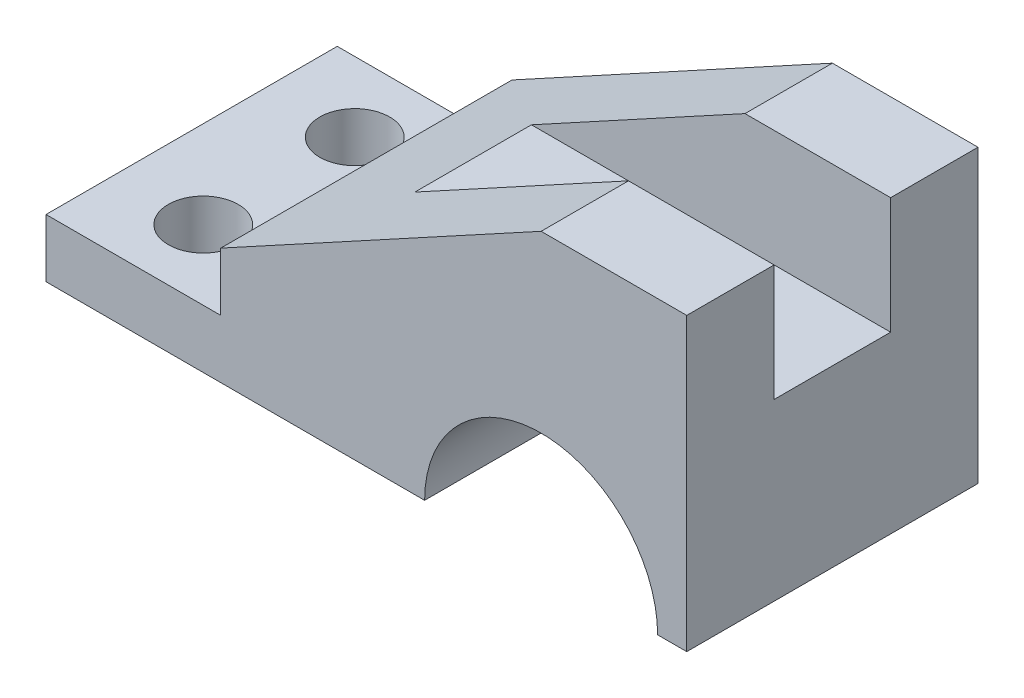
ISO-10303-21;
HEADER;
FILE_DESCRIPTION(('STEP AP214'),'2;1');
FILE_NAME('part.step','',(''),(''),'','','');
FILE_SCHEMA(('AUTOMOTIVE_DESIGN { 1 0 10303 214 1 1 1 1 }'));
ENDSEC;
DATA;
#1=APPLICATION_CONTEXT('core data for automotive mechanical design processes');
#2=APPLICATION_PROTOCOL_DEFINITION('international standard','automotive_design',2000,#1);
#3=PRODUCT_CONTEXT('',#1,'mechanical');
#4=PRODUCT('Part','Part','',(#3));
#5=PRODUCT_RELATED_PRODUCT_CATEGORY('part','',(#4));
#6=PRODUCT_DEFINITION_FORMATION('','',#4);
#7=PRODUCT_DEFINITION_CONTEXT('part definition',#1,'design');
#8=PRODUCT_DEFINITION('design','',#6,#7);
#9=PRODUCT_DEFINITION_SHAPE('','',#8);
#10=(LENGTH_UNIT() NAMED_UNIT(*) SI_UNIT(.MILLI.,.METRE.));
#11=(NAMED_UNIT(*) PLANE_ANGLE_UNIT() SI_UNIT($,.RADIAN.));
#12=(NAMED_UNIT(*) SI_UNIT($,.STERADIAN.) SOLID_ANGLE_UNIT());
#13=UNCERTAINTY_MEASURE_WITH_UNIT(LENGTH_MEASURE(1.E-05),#10,'distance_accuracy_value','');
#14=(GEOMETRIC_REPRESENTATION_CONTEXT(3) GLOBAL_UNCERTAINTY_ASSIGNED_CONTEXT((#13)) GLOBAL_UNIT_ASSIGNED_CONTEXT((#10,
#11,#12)) REPRESENTATION_CONTEXT('',''));
#15=CARTESIAN_POINT('',(0.,0.,0.));
#16=DIRECTION('',(0.,0.,1.));
#17=DIRECTION('',(1.,0.,0.));
#18=AXIS2_PLACEMENT_3D('',#15,#16,#17);
#19=CARTESIAN_POINT('',(110.,50.,50.));
#20=DIRECTION('',(0.,-1.,0.));
#21=DIRECTION('',(0.,0.,-1.));
#22=AXIS2_PLACEMENT_3D('',#19,#20,#21);
#23=PLANE('',#22);
#24=DIRECTION('',(0.,0.,-1.));
#25=VECTOR('',#24,1.);
#26=CARTESIAN_POINT('',(110.,50.,50.));
#27=LINE('',#26,#25);
#28=CARTESIAN_POINT('',(110.,50.,50.));
#29=VERTEX_POINT('',#28);
#30=CARTESIAN_POINT('',(110.,50.,35.));
#31=VERTEX_POINT('',#30);
#32=EDGE_CURVE('E174',#29,#31,#27,.T.);
#33=ORIENTED_EDGE('',*,*,#32,.T.);
#34=DIRECTION('',(1.,0.,0.));
#35=VECTOR('',#34,1.);
#36=CARTESIAN_POINT('',(85.,50.,35.));
#37=LINE('',#36,#35);
#38=CARTESIAN_POINT('',(85.,50.,35.));
#39=VERTEX_POINT('',#38);
#40=EDGE_CURVE('E220',#39,#31,#37,.T.);
#41=ORIENTED_EDGE('',*,*,#40,.F.);
#42=DIRECTION('',(0.,0.,-1.));
#43=VECTOR('',#42,1.);
#44=CARTESIAN_POINT('',(85.,50.,50.));
#45=LINE('',#44,#43);
#46=CARTESIAN_POINT('',(85.,50.,50.));
#47=VERTEX_POINT('',#46);
#48=EDGE_CURVE('E166',#47,#39,#45,.T.);
#49=ORIENTED_EDGE('',*,*,#48,.F.);
#50=DIRECTION('',(-1.,0.,0.));
#51=VECTOR('',#50,1.);
#52=CARTESIAN_POINT('',(110.,50.,50.));
#53=LINE('',#52,#51);
#54=EDGE_CURVE('E126',#29,#47,#53,.T.);
#55=ORIENTED_EDGE('',*,*,#54,.F.);
#56=EDGE_LOOP('',(#33,#41,#49,#55));
#57=FACE_BOUND('',#56,.T.);
#58=ADVANCED_FACE('F39',(#57),#23,.F.);
#59=CARTESIAN_POINT('',(0.,0.,50.));
#60=DIRECTION('',(1.,0.,0.));
#61=DIRECTION('',(0.,0.,-1.));
#62=AXIS2_PLACEMENT_3D('',#59,#60,#61);
#63=PLANE('',#62);
#64=DIRECTION('',(0.,-1.,0.));
#65=VECTOR('',#64,1.);
#66=CARTESIAN_POINT('',(0.,0.,0.));
#67=LINE('',#66,#65);
#68=CARTESIAN_POINT('',(0.,10.,0.));
#69=VERTEX_POINT('',#68);
#70=CARTESIAN_POINT('',(0.,0.,0.));
#71=VERTEX_POINT('',#70);
#72=EDGE_CURVE('E150',#69,#71,#67,.T.);
#73=ORIENTED_EDGE('',*,*,#72,.T.);
#74=DIRECTION('',(0.,0.,-1.));
#75=VECTOR('',#74,1.);
#76=CARTESIAN_POINT('',(0.,0.,50.));
#77=LINE('',#76,#75);
#78=CARTESIAN_POINT('',(0.,0.,50.));
#79=VERTEX_POINT('',#78);
#80=EDGE_CURVE('E11',#79,#71,#77,.T.);
#81=ORIENTED_EDGE('',*,*,#80,.F.);
#82=DIRECTION('',(0.,-1.,0.));
#83=VECTOR('',#82,1.);
#84=CARTESIAN_POINT('',(0.,0.,50.));
#85=LINE('',#84,#83);
#86=CARTESIAN_POINT('',(0.,10.,50.));
#87=VERTEX_POINT('',#86);
#88=EDGE_CURVE('E167',#87,#79,#85,.T.);
#89=ORIENTED_EDGE('',*,*,#88,.F.);
#90=DIRECTION('',(0.,0.,-1.));
#91=VECTOR('',#90,1.);
#92=CARTESIAN_POINT('',(0.,10.,50.));
#93=LINE('',#92,#91);
#94=EDGE_CURVE('E141',#87,#69,#93,.T.);
#95=ORIENTED_EDGE('',*,*,#94,.T.);
#96=EDGE_LOOP('',(#73,#81,#89,#95));
#97=FACE_BOUND('',#96,.T.);
#98=ADVANCED_FACE('F41',(#97),#63,.F.);
#99=CARTESIAN_POINT('',(0.,0.,50.));
#100=DIRECTION('',(0.,1.,0.));
#101=DIRECTION('',(0.,0.,1.));
#102=AXIS2_PLACEMENT_3D('',#99,#100,#101);
#103=PLANE('',#102);
#104=CARTESIAN_POINT('',(15.,0.,12.));
#105=DIRECTION('',(0.,1.,0.));
#106=DIRECTION('',(0.,0.,1.));
#107=AXIS2_PLACEMENT_3D('',#104,#105,#106);
#108=CIRCLE('',#107,6.);
#109=CARTESIAN_POINT('',(15.,0.,18.));
#110=VERTEX_POINT('',#109);
#111=EDGE_CURVE('E239',#110,#110,#108,.T.);
#112=ORIENTED_EDGE('',*,*,#111,.T.);
#113=EDGE_LOOP('',(#112));
#114=FACE_BOUND('',#113,.T.);
#115=CARTESIAN_POINT('',(15.,0.,38.));
#116=DIRECTION('',(0.,1.,0.));
#117=DIRECTION('',(0.,0.,1.));
#118=AXIS2_PLACEMENT_3D('',#115,#116,#117);
#119=CIRCLE('',#118,6.);
#120=CARTESIAN_POINT('',(15.,0.,44.));
#121=VERTEX_POINT('',#120);
#122=EDGE_CURVE('E242',#121,#121,#119,.T.);
#123=ORIENTED_EDGE('',*,*,#122,.T.);
#124=EDGE_LOOP('',(#123));
#125=FACE_BOUND('',#124,.T.);
#126=DIRECTION('',(1.,0.,0.));
#127=VECTOR('',#126,1.);
#128=CARTESIAN_POINT('',(0.,0.,0.));
#129=LINE('',#128,#127);
#130=CARTESIAN_POINT('',(65.,0.,0.));
#131=VERTEX_POINT('',#130);
#132=EDGE_CURVE('E147',#71,#131,#129,.T.);
#133=ORIENTED_EDGE('',*,*,#132,.T.);
#134=DIRECTION('',(0.,0.,-1.));
#135=VECTOR('',#134,1.);
#136=CARTESIAN_POINT('',(65.,0.,50.));
#137=LINE('',#136,#135);
#138=CARTESIAN_POINT('',(65.,0.,50.));
#139=VERTEX_POINT('',#138);
#140=EDGE_CURVE('E48',#139,#131,#137,.T.);
#141=ORIENTED_EDGE('',*,*,#140,.F.);
#142=DIRECTION('',(1.,0.,0.));
#143=VECTOR('',#142,1.);
#144=CARTESIAN_POINT('',(0.,0.,50.));
#145=LINE('',#144,#143);
#146=EDGE_CURVE('E103',#79,#139,#145,.T.);
#147=ORIENTED_EDGE('',*,*,#146,.F.);
#148=ORIENTED_EDGE('',*,*,#80,.T.);
#149=EDGE_LOOP('',(#133,#141,#147,#148));
#150=FACE_BOUND('',#149,.T.);
#151=ADVANCED_FACE('F252',(#114,#125,#150),#103,.F.);
#152=CARTESIAN_POINT('',(85.,0.,50.));
#153=DIRECTION('',(0.,0.,-1.));
#154=DIRECTION('',(-1.,0.,0.));
#155=AXIS2_PLACEMENT_3D('',#152,#153,#154);
#156=CYLINDRICAL_SURFACE('',#155,20.);
#157=CARTESIAN_POINT('',(85.,0.,0.));
#158=DIRECTION('',(0.,0.,-1.));
#159=DIRECTION('',(1.,0.,0.));
#160=AXIS2_PLACEMENT_3D('',#157,#158,#159);
#161=CIRCLE('',#160,20.);
#162=CARTESIAN_POINT('',(105.,0.,0.));
#163=VERTEX_POINT('',#162);
#164=EDGE_CURVE('E153',#131,#163,#161,.T.);
#165=ORIENTED_EDGE('',*,*,#164,.T.);
#166=DIRECTION('',(0.,0.,-1.));
#167=VECTOR('',#166,1.);
#168=CARTESIAN_POINT('',(105.,0.,50.));
#169=LINE('',#168,#167);
#170=CARTESIAN_POINT('',(105.,0.,50.));
#171=VERTEX_POINT('',#170);
#172=EDGE_CURVE('E177',#171,#163,#169,.T.);
#173=ORIENTED_EDGE('',*,*,#172,.F.);
#174=CARTESIAN_POINT('',(85.,0.,50.));
#175=DIRECTION('',(0.,0.,-1.));
#176=DIRECTION('',(1.,0.,0.));
#177=AXIS2_PLACEMENT_3D('',#174,#175,#176);
#178=CIRCLE('',#177,20.);
#179=EDGE_CURVE('E188',#139,#171,#178,.T.);
#180=ORIENTED_EDGE('',*,*,#179,.F.);
#181=ORIENTED_EDGE('',*,*,#140,.T.);
#182=EDGE_LOOP('',(#165,#173,#180,#181));
#183=FACE_BOUND('',#182,.T.);
#184=ADVANCED_FACE('F184',(#183),#156,.F.);
#185=CARTESIAN_POINT('',(105.,0.,50.));
#186=DIRECTION('',(0.,1.,0.));
#187=DIRECTION('',(0.,0.,1.));
#188=AXIS2_PLACEMENT_3D('',#185,#186,#187);
#189=PLANE('',#188);
#190=DIRECTION('',(1.,0.,0.));
#191=VECTOR('',#190,1.);
#192=CARTESIAN_POINT('',(105.,0.,0.));
#193=LINE('',#192,#191);
#194=CARTESIAN_POINT('',(110.,0.,0.));
#195=VERTEX_POINT('',#194);
#196=EDGE_CURVE('E154',#163,#195,#193,.T.);
#197=ORIENTED_EDGE('',*,*,#196,.T.);
#198=DIRECTION('',(0.,0.,-1.));
#199=VECTOR('',#198,1.);
#200=CARTESIAN_POINT('',(110.,0.,50.));
#201=LINE('',#200,#199);
#202=CARTESIAN_POINT('',(110.,0.,50.));
#203=VERTEX_POINT('',#202);
#204=EDGE_CURVE('E171',#203,#195,#201,.T.);
#205=ORIENTED_EDGE('',*,*,#204,.F.);
#206=DIRECTION('',(1.,0.,0.));
#207=VECTOR('',#206,1.);
#208=CARTESIAN_POINT('',(105.,0.,50.));
#209=LINE('',#208,#207);
#210=EDGE_CURVE('E202',#171,#203,#209,.T.);
#211=ORIENTED_EDGE('',*,*,#210,.F.);
#212=ORIENTED_EDGE('',*,*,#172,.T.);
#213=EDGE_LOOP('',(#197,#205,#211,#212));
#214=FACE_BOUND('',#213,.T.);
#215=ADVANCED_FACE('F191',(#214),#189,.F.);
#216=CARTESIAN_POINT('',(110.,0.,50.));
#217=DIRECTION('',(-1.,0.,0.));
#218=DIRECTION('',(0.,0.,1.));
#219=AXIS2_PLACEMENT_3D('',#216,#217,#218);
#220=PLANE('',#219);
#221=DIRECTION('',(0.,0.,-1.));
#222=VECTOR('',#221,1.);
#223=CARTESIAN_POINT('',(110.,30.,15.));
#224=LINE('',#223,#222);
#225=CARTESIAN_POINT('',(110.,30.,35.));
#226=VERTEX_POINT('',#225);
#227=CARTESIAN_POINT('',(110.,30.,15.));
#228=VERTEX_POINT('',#227);
#229=EDGE_CURVE('E219',#226,#228,#224,.T.);
#230=ORIENTED_EDGE('',*,*,#229,.F.);
#231=DIRECTION('',(0.,1.,0.));
#232=VECTOR('',#231,1.);
#233=CARTESIAN_POINT('',(110.,30.,35.));
#234=LINE('',#233,#232);
#235=EDGE_CURVE('E151',#226,#31,#234,.T.);
#236=ORIENTED_EDGE('',*,*,#235,.T.);
#237=ORIENTED_EDGE('',*,*,#32,.F.);
#238=DIRECTION('',(0.,1.,0.));
#239=VECTOR('',#238,1.);
#240=CARTESIAN_POINT('',(110.,0.,50.));
#241=LINE('',#240,#239);
#242=EDGE_CURVE('E201',#203,#29,#241,.T.);
#243=ORIENTED_EDGE('',*,*,#242,.F.);
#244=ORIENTED_EDGE('',*,*,#204,.T.);
#245=DIRECTION('',(0.,1.,0.));
#246=VECTOR('',#245,1.);
#247=CARTESIAN_POINT('',(110.,0.,0.));
#248=LINE('',#247,#246);
#249=CARTESIAN_POINT('',(110.,50.,0.));
#250=VERTEX_POINT('',#249);
#251=EDGE_CURVE('E160',#195,#250,#248,.T.);
#252=ORIENTED_EDGE('',*,*,#251,.T.);
#253=CARTESIAN_POINT('',(110.,50.,15.));
#254=VERTEX_POINT('',#253);
#255=EDGE_CURVE('E173',#254,#250,#27,.T.);
#256=ORIENTED_EDGE('',*,*,#255,.F.);
#257=DIRECTION('',(0.,1.,0.));
#258=VECTOR('',#257,1.);
#259=CARTESIAN_POINT('',(110.,30.,15.));
#260=LINE('',#259,#258);
#261=EDGE_CURVE('E215',#228,#254,#260,.T.);
#262=ORIENTED_EDGE('',*,*,#261,.F.);
#263=EDGE_LOOP('',(#230,#236,#237,#243,#244,#252,#256,#262));
#264=FACE_BOUND('',#263,.T.);
#265=ADVANCED_FACE('F199',(#264),#220,.F.);
#266=CARTESIAN_POINT('',(85.,50.,15.));
#267=VERTEX_POINT('',#266);
#268=CARTESIAN_POINT('',(85.,50.,0.));
#269=VERTEX_POINT('',#268);
#270=EDGE_CURVE('E137',#267,#269,#45,.T.);
#271=ORIENTED_EDGE('',*,*,#270,.F.);
#272=DIRECTION('',(-1.,0.,0.));
#273=VECTOR('',#272,1.);
#274=CARTESIAN_POINT('',(85.,50.,15.));
#275=LINE('',#274,#273);
#276=EDGE_CURVE('E222',#254,#267,#275,.T.);
#277=ORIENTED_EDGE('',*,*,#276,.F.);
#278=ORIENTED_EDGE('',*,*,#255,.T.);
#279=DIRECTION('',(-1.,0.,0.));
#280=VECTOR('',#279,1.);
#281=CARTESIAN_POINT('',(110.,50.,0.));
#282=LINE('',#281,#280);
#283=EDGE_CURVE('E159',#250,#269,#282,.T.);
#284=ORIENTED_EDGE('',*,*,#283,.T.);
#285=EDGE_LOOP('',(#271,#277,#278,#284));
#286=FACE_BOUND('',#285,.T.);
#287=ADVANCED_FACE('F284',(#286),#23,.F.);
#288=CARTESIAN_POINT('',(30.,20.,50.));
#289=DIRECTION('',(0.478852130680573,-0.877895572914384,0.));
#290=DIRECTION('',(0.877895572914384,0.478852130680573,0.));
#291=AXIS2_PLACEMENT_3D('',#288,#289,#290);
#292=PLANE('',#291);
#293=DIRECTION('',(0.,0.,-1.));
#294=VECTOR('',#293,1.);
#295=CARTESIAN_POINT('',(48.3333333333333,30.,50.));
#296=LINE('',#295,#294);
#297=CARTESIAN_POINT('',(48.3333333333333,30.,35.));
#298=VERTEX_POINT('',#297);
#299=CARTESIAN_POINT('',(48.3333333333333,30.,15.));
#300=VERTEX_POINT('',#299);
#301=EDGE_CURVE('E235',#298,#300,#296,.T.);
#302=ORIENTED_EDGE('',*,*,#301,.T.);
#303=DIRECTION('',(0.877895572914384,0.478852130680573,0.));
#304=VECTOR('',#303,1.);
#305=CARTESIAN_POINT('',(30.,20.,15.));
#306=LINE('',#305,#304);
#307=EDGE_CURVE('E221',#300,#267,#306,.T.);
#308=ORIENTED_EDGE('',*,*,#307,.T.);
#309=ORIENTED_EDGE('',*,*,#270,.T.);
#310=DIRECTION('',(-0.877895572914384,-0.478852130680573,0.));
#311=VECTOR('',#310,1.);
#312=CARTESIAN_POINT('',(30.,20.,0.));
#313=LINE('',#312,#311);
#314=CARTESIAN_POINT('',(30.,20.,0.));
#315=VERTEX_POINT('',#314);
#316=EDGE_CURVE('E139',#269,#315,#313,.T.);
#317=ORIENTED_EDGE('',*,*,#316,.T.);
#318=DIRECTION('',(0.,0.,-1.));
#319=VECTOR('',#318,1.);
#320=CARTESIAN_POINT('',(30.,20.,50.));
#321=LINE('',#320,#319);
#322=CARTESIAN_POINT('',(30.,20.,50.));
#323=VERTEX_POINT('',#322);
#324=EDGE_CURVE('E132',#323,#315,#321,.T.);
#325=ORIENTED_EDGE('',*,*,#324,.F.);
#326=DIRECTION('',(-0.877895572914384,-0.478852130680573,0.));
#327=VECTOR('',#326,1.);
#328=CARTESIAN_POINT('',(30.,20.,50.));
#329=LINE('',#328,#327);
#330=EDGE_CURVE('E124',#47,#323,#329,.T.);
#331=ORIENTED_EDGE('',*,*,#330,.F.);
#332=ORIENTED_EDGE('',*,*,#48,.T.);
#333=DIRECTION('',(-0.877895572914384,-0.478852130680573,0.));
#334=VECTOR('',#333,1.);
#335=CARTESIAN_POINT('',(30.,20.,35.));
#336=LINE('',#335,#334);
#337=EDGE_CURVE('E237',#39,#298,#336,.T.);
#338=ORIENTED_EDGE('',*,*,#337,.T.);
#339=EDGE_LOOP('',(#302,#308,#309,#317,#325,#331,#332,#338));
#340=FACE_BOUND('',#339,.T.);
#341=ADVANCED_FACE('F131',(#340),#292,.F.);
#342=CARTESIAN_POINT('',(30.,10.,50.));
#343=DIRECTION('',(1.,0.,0.));
#344=DIRECTION('',(0.,0.,-1.));
#345=AXIS2_PLACEMENT_3D('',#342,#343,#344);
#346=PLANE('',#345);
#347=DIRECTION('',(0.,-1.,0.));
#348=VECTOR('',#347,1.);
#349=CARTESIAN_POINT('',(30.,10.,0.));
#350=LINE('',#349,#348);
#351=CARTESIAN_POINT('',(30.,10.,0.));
#352=VERTEX_POINT('',#351);
#353=EDGE_CURVE('E90',#315,#352,#350,.T.);
#354=ORIENTED_EDGE('',*,*,#353,.T.);
#355=DIRECTION('',(0.,0.,-1.));
#356=VECTOR('',#355,1.);
#357=CARTESIAN_POINT('',(30.,10.,50.));
#358=LINE('',#357,#356);
#359=CARTESIAN_POINT('',(30.,10.,50.));
#360=VERTEX_POINT('',#359);
#361=EDGE_CURVE('E140',#360,#352,#358,.T.);
#362=ORIENTED_EDGE('',*,*,#361,.F.);
#363=DIRECTION('',(0.,-1.,0.));
#364=VECTOR('',#363,1.);
#365=CARTESIAN_POINT('',(30.,10.,50.));
#366=LINE('',#365,#364);
#367=EDGE_CURVE('E127',#323,#360,#366,.T.);
#368=ORIENTED_EDGE('',*,*,#367,.F.);
#369=ORIENTED_EDGE('',*,*,#324,.T.);
#370=EDGE_LOOP('',(#354,#362,#368,#369));
#371=FACE_BOUND('',#370,.T.);
#372=ADVANCED_FACE('F143',(#371),#346,.F.);
#373=CARTESIAN_POINT('',(0.,10.,50.));
#374=DIRECTION('',(0.,-1.,0.));
#375=DIRECTION('',(0.,0.,-1.));
#376=AXIS2_PLACEMENT_3D('',#373,#374,#375);
#377=PLANE('',#376);
#378=CARTESIAN_POINT('',(15.,10.,12.));
#379=DIRECTION('',(0.,1.,0.));
#380=DIRECTION('',(0.,0.,1.));
#381=AXIS2_PLACEMENT_3D('',#378,#379,#380);
#382=CIRCLE('',#381,6.);
#383=CARTESIAN_POINT('',(15.,10.,18.));
#384=VERTEX_POINT('',#383);
#385=EDGE_CURVE('E248',#384,#384,#382,.T.);
#386=ORIENTED_EDGE('',*,*,#385,.F.);
#387=EDGE_LOOP('',(#386));
#388=FACE_BOUND('',#387,.T.);
#389=CARTESIAN_POINT('',(15.,10.,38.));
#390=DIRECTION('',(0.,1.,0.));
#391=DIRECTION('',(0.,0.,1.));
#392=AXIS2_PLACEMENT_3D('',#389,#390,#391);
#393=CIRCLE('',#392,6.);
#394=CARTESIAN_POINT('',(15.,10.,44.));
#395=VERTEX_POINT('',#394);
#396=EDGE_CURVE('E238',#395,#395,#393,.T.);
#397=ORIENTED_EDGE('',*,*,#396,.F.);
#398=EDGE_LOOP('',(#397));
#399=FACE_BOUND('',#398,.T.);
#400=DIRECTION('',(-1.,0.,0.));
#401=VECTOR('',#400,1.);
#402=CARTESIAN_POINT('',(0.,10.,0.));
#403=LINE('',#402,#401);
#404=EDGE_CURVE('E92',#352,#69,#403,.T.);
#405=ORIENTED_EDGE('',*,*,#404,.T.);
#406=ORIENTED_EDGE('',*,*,#94,.F.);
#407=DIRECTION('',(-1.,0.,0.));
#408=VECTOR('',#407,1.);
#409=CARTESIAN_POINT('',(0.,10.,50.));
#410=LINE('',#409,#408);
#411=EDGE_CURVE('E57',#360,#87,#410,.T.);
#412=ORIENTED_EDGE('',*,*,#411,.F.);
#413=ORIENTED_EDGE('',*,*,#361,.T.);
#414=EDGE_LOOP('',(#405,#406,#412,#413));
#415=FACE_BOUND('',#414,.T.);
#416=ADVANCED_FACE('F265',(#388,#399,#415),#377,.F.);
#417=CARTESIAN_POINT('',(85.,0.,50.));
#418=DIRECTION('',(0.,0.,1.));
#419=DIRECTION('',(1.,0.,0.));
#420=AXIS2_PLACEMENT_3D('',#417,#418,#419);
#421=PLANE('',#420);
#422=ORIENTED_EDGE('',*,*,#88,.T.);
#423=ORIENTED_EDGE('',*,*,#146,.T.);
#424=ORIENTED_EDGE('',*,*,#179,.T.);
#425=ORIENTED_EDGE('',*,*,#210,.T.);
#426=ORIENTED_EDGE('',*,*,#242,.T.);
#427=ORIENTED_EDGE('',*,*,#54,.T.);
#428=ORIENTED_EDGE('',*,*,#330,.T.);
#429=ORIENTED_EDGE('',*,*,#367,.T.);
#430=ORIENTED_EDGE('',*,*,#411,.T.);
#431=EDGE_LOOP('',(#422,#423,#424,#425,#426,#427,#428,#429,#430));
#432=FACE_BOUND('',#431,.T.);
#433=ADVANCED_FACE('F125',(#432),#421,.T.);
#434=CARTESIAN_POINT('',(85.,0.,0.));
#435=DIRECTION('',(0.,0.,1.));
#436=DIRECTION('',(1.,0.,0.));
#437=AXIS2_PLACEMENT_3D('',#434,#435,#436);
#438=PLANE('',#437);
#439=ORIENTED_EDGE('',*,*,#72,.F.);
#440=ORIENTED_EDGE('',*,*,#404,.F.);
#441=ORIENTED_EDGE('',*,*,#353,.F.);
#442=ORIENTED_EDGE('',*,*,#316,.F.);
#443=ORIENTED_EDGE('',*,*,#283,.F.);
#444=ORIENTED_EDGE('',*,*,#251,.F.);
#445=ORIENTED_EDGE('',*,*,#196,.F.);
#446=ORIENTED_EDGE('',*,*,#164,.F.);
#447=ORIENTED_EDGE('',*,*,#132,.F.);
#448=EDGE_LOOP('',(#439,#440,#441,#442,#443,#444,#445,#446,#447));
#449=FACE_BOUND('',#448,.T.);
#450=ADVANCED_FACE('F186',(#449),#438,.F.);
#451=CARTESIAN_POINT('',(85.,30.,35.));
#452=DIRECTION('',(0.,0.,1.));
#453=DIRECTION('',(1.,0.,0.));
#454=AXIS2_PLACEMENT_3D('',#451,#452,#453);
#455=PLANE('',#454);
#456=ORIENTED_EDGE('',*,*,#40,.T.);
#457=ORIENTED_EDGE('',*,*,#235,.F.);
#458=DIRECTION('',(1.,0.,0.));
#459=VECTOR('',#458,1.);
#460=CARTESIAN_POINT('',(85.,30.,35.));
#461=LINE('',#460,#459);
#462=EDGE_CURVE('E214',#298,#226,#461,.T.);
#463=ORIENTED_EDGE('',*,*,#462,.F.);
#464=ORIENTED_EDGE('',*,*,#337,.F.);
#465=EDGE_LOOP('',(#456,#457,#463,#464));
#466=FACE_BOUND('',#465,.T.);
#467=ADVANCED_FACE('F317',(#466),#455,.F.);
#468=CARTESIAN_POINT('',(85.,30.,15.));
#469=DIRECTION('',(0.,0.,-1.));
#470=DIRECTION('',(-1.,0.,0.));
#471=AXIS2_PLACEMENT_3D('',#468,#469,#470);
#472=PLANE('',#471);
#473=ORIENTED_EDGE('',*,*,#276,.T.);
#474=ORIENTED_EDGE('',*,*,#307,.F.);
#475=DIRECTION('',(-1.,0.,0.));
#476=VECTOR('',#475,1.);
#477=CARTESIAN_POINT('',(85.,30.,15.));
#478=LINE('',#477,#476);
#479=EDGE_CURVE('E229',#228,#300,#478,.T.);
#480=ORIENTED_EDGE('',*,*,#479,.F.);
#481=ORIENTED_EDGE('',*,*,#261,.T.);
#482=EDGE_LOOP('',(#473,#474,#480,#481));
#483=FACE_BOUND('',#482,.T.);
#484=ADVANCED_FACE('F274',(#483),#472,.F.);
#485=CARTESIAN_POINT('',(0.,30.,0.));
#486=DIRECTION('',(0.,1.,0.));
#487=DIRECTION('',(0.,0.,1.));
#488=AXIS2_PLACEMENT_3D('',#485,#486,#487);
#489=PLANE('',#488);
#490=ORIENTED_EDGE('',*,*,#229,.T.);
#491=ORIENTED_EDGE('',*,*,#479,.T.);
#492=ORIENTED_EDGE('',*,*,#301,.F.);
#493=ORIENTED_EDGE('',*,*,#462,.T.);
#494=EDGE_LOOP('',(#490,#491,#492,#493));
#495=FACE_BOUND('',#494,.T.);
#496=ADVANCED_FACE('F267',(#495),#489,.T.);
#497=CARTESIAN_POINT('',(15.,0.,38.));
#498=DIRECTION('',(0.,1.,0.));
#499=DIRECTION('',(0.,0.,1.));
#500=AXIS2_PLACEMENT_3D('',#497,#498,#499);
#501=CYLINDRICAL_SURFACE('',#500,6.);
#502=ORIENTED_EDGE('',*,*,#122,.F.);
#503=EDGE_LOOP('',(#502));
#504=FACE_BOUND('',#503,.T.);
#505=ORIENTED_EDGE('',*,*,#396,.T.);
#506=EDGE_LOOP('',(#505));
#507=FACE_BOUND('',#506,.T.);
#508=ADVANCED_FACE('F256',(#504,#507),#501,.F.);
#509=CARTESIAN_POINT('',(15.,0.,12.));
#510=DIRECTION('',(0.,1.,0.));
#511=DIRECTION('',(0.,0.,1.));
#512=AXIS2_PLACEMENT_3D('',#509,#510,#511);
#513=CYLINDRICAL_SURFACE('',#512,6.);
#514=ORIENTED_EDGE('',*,*,#111,.F.);
#515=EDGE_LOOP('',(#514));
#516=FACE_BOUND('',#515,.T.);
#517=ORIENTED_EDGE('',*,*,#385,.T.);
#518=EDGE_LOOP('',(#517));
#519=FACE_BOUND('',#518,.T.);
#520=ADVANCED_FACE('F254',(#516,#519),#513,.F.);
#521=CLOSED_SHELL('',(#58,#98,#151,#184,#215,#265,#287,#341,#372,#416,#433,#450,#467,#484,#496,
#508,#520));
#522=MANIFOLD_SOLID_BREP('B2',#521);
#523=ADVANCED_BREP_SHAPE_REPRESENTATION('',(#18,#522),#14);
#524=SHAPE_DEFINITION_REPRESENTATION(#9,#523);
ENDSEC;
END-ISO-10303-21;
